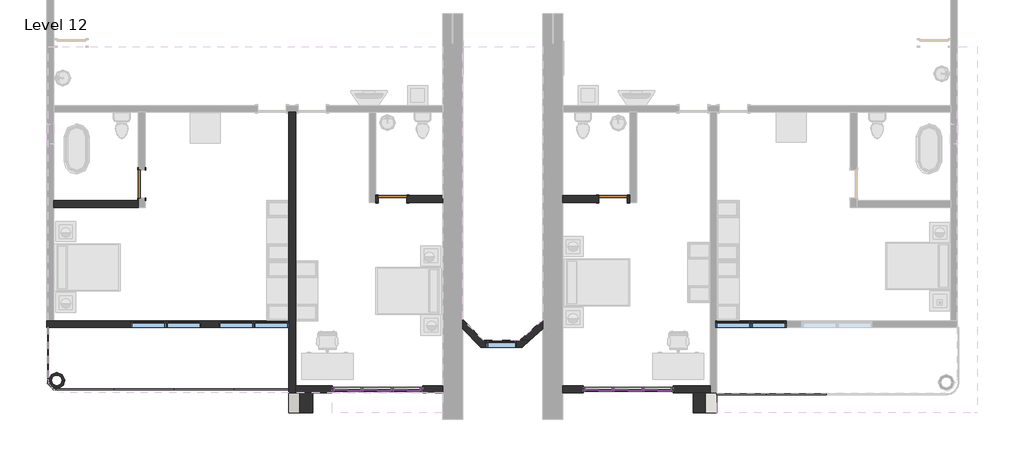
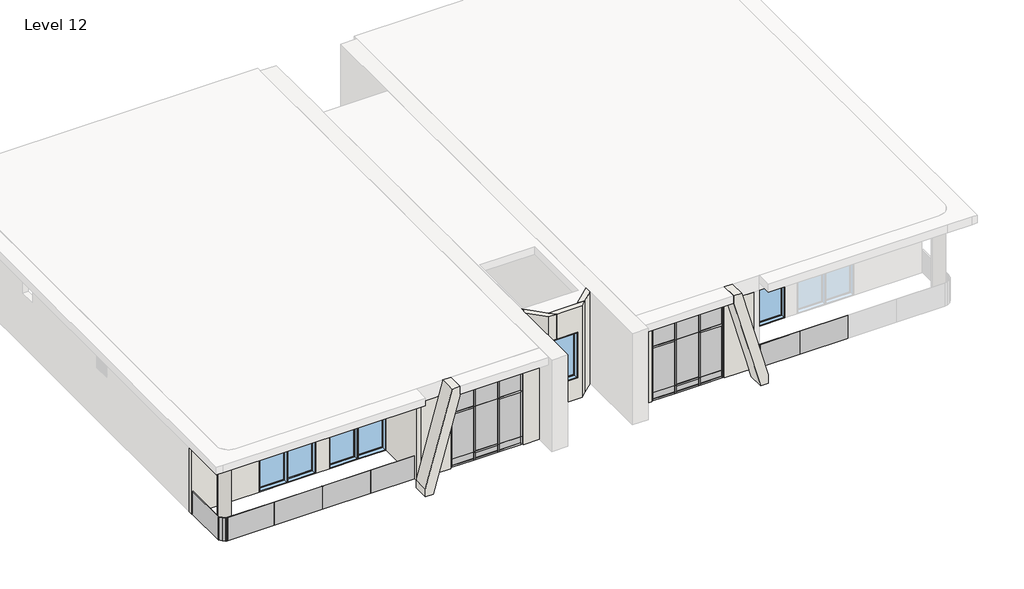
# One storey, part 1 of 3: 42 members, 29 plates, 16 walls, 7 windows, 3 doors.
"""IFC4 building model written with IfcOpenShell, lengths in millimetres."""

from ifc_helpers import new_model, si_unit, point, frame, frame_2d, origin, place, context, project, spatial, polyline, circle_curve, trimmed, segment, composite_curve, outline, extrude, faceted_brep, transform, mapped, element, save
from components import door_2703ae13, door_10fd3a06, member_c17f1be2, member_ad567e07, member_d2e7e466, member_7db1855a, member_75d1e245, member_d60e8053, member_3c3dc66a, member_2fae0574, member_410c6227, member_73c23c35, system_panel_glazed_38d54ecf, system_panel_glazed_fbb6c980, system_panel_glazed_4137532c, system_panel_glazed_6230de04, system_panel_glazed_a79f7f85, system_panel_glazed_9a5ea490, system_panel_glazed_95be5de7, system_panel_glazed_ffe51582, system_panel_glazed_8f95e3f6, system_panel_glazed_836907cd, system_panel_glazed_688a65a2, system_panel_glazed_c1a1c740, system_panel_glazed_22bcd51f, system_panel_glazed_b07a1a35, window_9a779fa2, window_1a213a25

model = new_model("IFC4")

# Units and contexts
model_context = context("Model", 3, world=origin())
ifc_project = project(units=[si_unit("LENGTHUNIT", "METRE", prefix="MILLI")], contexts=[model_context])

# Site, building, storey
site = spatial("IfcSite", under=ifc_project)
building = spatial("IfcBuilding", under=site)
storey = spatial("IfcBuildingStorey", under=building, Name="Level 12", Elevation=40233.6)

# Doors
placement = place(None, origin())
door_shape = door_2703ae13(model_context)
element("IfcDoor", 1, ObjectType="Door-Single-Panel.0001 : 34\" x 80\"", at=placement, inside=storey, context=model_context, shape_type="MappedRepresentation", body=[
    mapped(door_shape, transform((-15765.9987704, -441.9241442, 40233.6), x_axis=(0.0, -1.0, 0.0), y_axis=(1.0, 0.0, 0.0), z_axis=(0.0, 0.0, 1.0))),
])
element("IfcDoor", 2, ObjectType="Door-Single-Panel.0001 : 34\" x 80\"", at=placement, inside=storey, context=model_context, shape_type="MappedRepresentation", body=[
    mapped(door_shape, transform((-8145.9987704, -899.1241442, 40233.6), x_axis=(-1.0, 0.0, 0.0), y_axis=(0.0, -1.0, 0.0), z_axis=(0.0, 0.0, 1.0))),
])
door_2_shape = door_10fd3a06(model_context)
element("IfcDoor", 3, ObjectType="Door-Single-Panel.0001 : 34\" x 80\"", at=placement, inside=storey, context=model_context, shape_type="MappedRepresentation", body=[
    mapped(door_2_shape, transform((-1440.3987704, -899.1241442, 40233.6), x_axis=(1.0, 0.0, 0.0), y_axis=(0.0, 1.0, 0.0), z_axis=(0.0, 0.0, 1.0))),
])

# Members
member_shape = member_c17f1be2(model_context)
element("IfcMember", 4, ObjectType="Rectangular Mullion : 2.5\" x 5\" rectangular", at=placement, inside=storey, context=model_context, shape_type="MappedRepresentation", body=[
    mapped(member_shape, transform((-9911.2987704, -6690.3241442, 43281.6), x_axis=(0.0, 0.0, 1.0), y_axis=(0.0, 1.0, 0.0), z_axis=(-1.0, 0.0, 0.0))),
])
element("IfcMember", 5, ObjectType="Rectangular Mullion : 2.5\" x 5\" rectangular", at=placement, inside=storey, context=model_context, shape_type="MappedRepresentation", body=[
    mapped(member_shape, transform((-8114.2487704, -6690.3241442, 43281.6), x_axis=(0.0, 0.0, 1.0), y_axis=(0.0, 1.0, 0.0), z_axis=(-1.0, 0.0, 0.0))),
])
element("IfcMember", 6, ObjectType="Rectangular Mullion : 2.5\" x 5\" rectangular", at=placement, inside=storey, context=model_context, shape_type="MappedRepresentation", body=[
    mapped(member_shape, transform((-2291.2987704, -6690.3241442, 43281.6), x_axis=(0.0, 0.0, 1.0), y_axis=(0.0, 1.0, 0.0), z_axis=(-1.0, 0.0, 0.0))),
])
element("IfcMember", 7, ObjectType="Rectangular Mullion : 2.5\" x 5\" rectangular", at=placement, inside=storey, context=model_context, shape_type="MappedRepresentation", body=[
    mapped(member_shape, transform((-494.2487704, -6690.3241442, 43281.6), x_axis=(0.0, 0.0, 1.0), y_axis=(0.0, 1.0, 0.0), z_axis=(-1.0, 0.0, 0.0))),
])
element("IfcMember", 8, ObjectType="Rectangular Mullion : 2.5\" x 5\" rectangular", at=placement, inside=storey, context=model_context, shape_type="MappedRepresentation", body=[
    mapped(member_shape, transform((-7295.0987704, -6690.3241442, 40233.6), x_axis=(0.0, 0.0, -1.0), y_axis=(0.0, 1.0, 0.0), z_axis=(1.0, 0.0, 0.0))),
])
element("IfcMember", 9, ObjectType="Rectangular Mullion : 2.5\" x 5\" rectangular", at=placement, inside=storey, context=model_context, shape_type="MappedRepresentation", body=[
    mapped(member_shape, transform((-9092.1487704, -6690.3241442, 40233.6), x_axis=(0.0, 0.0, -1.0), y_axis=(0.0, 1.0, 0.0), z_axis=(1.0, 0.0, 0.0))),
])
element("IfcMember", 10, ObjectType="Rectangular Mullion : 2.5\" x 5\" rectangular", at=placement, inside=storey, context=model_context, shape_type="MappedRepresentation", body=[
    mapped(member_shape, transform((324.9012296, -6690.3241442, 40233.6), x_axis=(0.0, 0.0, -1.0), y_axis=(0.0, 1.0, 0.0), z_axis=(1.0, 0.0, 0.0))),
])
element("IfcMember", 11, ObjectType="Rectangular Mullion : 2.5\" x 5\" rectangular", at=placement, inside=storey, context=model_context, shape_type="MappedRepresentation", body=[
    mapped(member_shape, transform((-1472.1487704, -6690.3241442, 40233.6), x_axis=(0.0, 0.0, -1.0), y_axis=(0.0, 1.0, 0.0), z_axis=(1.0, 0.0, 0.0))),
])
member_2_shape = member_ad567e07(model_context)
element("IfcMember", 12, ObjectType="Rectangular Mullion : 2.5\" x 5\" rectangular", at=placement, inside=storey, context=model_context, shape_type="MappedRepresentation", body=[
    mapped(member_2_shape, transform((-8114.2487704, -6690.3241442, 42367.2), x_axis=(0.0, 0.0, 1.0), y_axis=(0.0, 1.0, 0.0), z_axis=(-1.0, 0.0, 0.0))),
])
element("IfcMember", 13, ObjectType="Rectangular Mullion : 2.5\" x 5\" rectangular", at=placement, inside=storey, context=model_context, shape_type="MappedRepresentation", body=[
    mapped(member_2_shape, transform((-9911.2987704, -6690.3241442, 42367.2), x_axis=(0.0, 0.0, 1.0), y_axis=(0.0, 1.0, 0.0), z_axis=(-1.0, 0.0, 0.0))),
])
element("IfcMember", 14, ObjectType="Rectangular Mullion : 2.5\" x 5\" rectangular", at=placement, inside=storey, context=model_context, shape_type="MappedRepresentation", body=[
    mapped(member_2_shape, transform((-494.2487704, -6690.3241442, 42367.2), x_axis=(0.0, 0.0, 1.0), y_axis=(0.0, 1.0, 0.0), z_axis=(-1.0, 0.0, 0.0))),
])
element("IfcMember", 15, ObjectType="Rectangular Mullion : 2.5\" x 5\" rectangular", at=placement, inside=storey, context=model_context, shape_type="MappedRepresentation", body=[
    mapped(member_2_shape, transform((-2291.2987704, -6690.3241442, 42367.2), x_axis=(0.0, 0.0, 1.0), y_axis=(0.0, 1.0, 0.0), z_axis=(-1.0, 0.0, 0.0))),
])
member_3_shape = member_d2e7e466(model_context)
element("IfcMember", 16, ObjectType="Rectangular Mullion : 2.5\" x 5\" rectangular", at=placement, inside=storey, context=model_context, shape_type="MappedRepresentation", body=[
    mapped(member_3_shape, transform((-8177.7487704, -6690.3241442, 40233.6), x_axis=(0.0, 0.0, -1.0), y_axis=(0.0, 1.0, 0.0), z_axis=(1.0, 0.0, 0.0))),
])
element("IfcMember", 17, ObjectType="Rectangular Mullion : 2.5\" x 5\" rectangular", at=placement, inside=storey, context=model_context, shape_type="MappedRepresentation", body=[
    mapped(member_3_shape, transform((-557.7487704, -6690.3241442, 40233.6), x_axis=(0.0, 0.0, -1.0), y_axis=(0.0, 1.0, 0.0), z_axis=(1.0, 0.0, 0.0))),
])
member_4_shape = member_7db1855a(model_context)
element("IfcMember", 18, ObjectType="Rectangular Mullion : 2.5\" x 5\" rectangular", at=placement, inside=storey, context=model_context, shape_type="MappedRepresentation", body=[
    mapped(member_4_shape, transform((-9028.6487704, -6690.3241442, 40538.4), x_axis=(0.0, 0.0, 1.0), y_axis=(0.0, 1.0, 0.0), z_axis=(-1.0, 0.0, 0.0))),
])
element("IfcMember", 19, ObjectType="Rectangular Mullion : 2.5\" x 5\" rectangular", at=placement, inside=storey, context=model_context, shape_type="MappedRepresentation", body=[
    mapped(member_4_shape, transform((-1408.6487704, -6690.3241442, 40538.4), x_axis=(0.0, 0.0, 1.0), y_axis=(0.0, 1.0, 0.0), z_axis=(-1.0, 0.0, 0.0))),
])
element("IfcMember", 20, ObjectType="Rectangular Mullion : 2.5\" x 5\" rectangular", at=placement, inside=storey, context=model_context, shape_type="MappedRepresentation", body=[
    mapped(member_3_shape, transform((-9028.6487704, -6690.3241442, 43281.6), x_axis=(0.0, 0.0, 1.0), y_axis=(0.0, 1.0, 0.0), z_axis=(-1.0, 0.0, 0.0))),
])
element("IfcMember", 21, ObjectType="Rectangular Mullion : 2.5\" x 5\" rectangular", at=placement, inside=storey, context=model_context, shape_type="MappedRepresentation", body=[
    mapped(member_3_shape, transform((-1408.6487704, -6690.3241442, 43281.6), x_axis=(0.0, 0.0, 1.0), y_axis=(0.0, 1.0, 0.0), z_axis=(-1.0, 0.0, 0.0))),
])
member_5_shape = member_75d1e245(model_context)
element("IfcMember", 22, ObjectType="Rectangular Mullion : 2.5\" x 5\" rectangular", at=placement, inside=storey, context=model_context, shape_type="MappedRepresentation", body=[
    mapped(member_5_shape, transform((-8145.9987704, -6690.3241442, 40233.6), x_axis=(-1.0, 0.0, 0.0), y_axis=(0.0, 1.0, 0.0), z_axis=(0.0, 0.0, -1.0))),
])
element("IfcMember", 23, ObjectType="Rectangular Mullion : 2.5\" x 5\" rectangular", at=placement, inside=storey, context=model_context, shape_type="MappedRepresentation", body=[
    mapped(member_5_shape, transform((-9060.3987704, -6690.3241442, 40233.6), x_axis=(-1.0, 0.0, 0.0), y_axis=(0.0, 1.0, 0.0), z_axis=(0.0, 0.0, -1.0))),
])
element("IfcMember", 24, ObjectType="Rectangular Mullion : 2.5\" x 5\" rectangular", at=placement, inside=storey, context=model_context, shape_type="MappedRepresentation", body=[
    mapped(member_5_shape, transform((-525.9987704, -6690.3241442, 40233.6), x_axis=(-1.0, 0.0, 0.0), y_axis=(0.0, 1.0, 0.0), z_axis=(0.0, 0.0, -1.0))),
])
element("IfcMember", 25, ObjectType="Rectangular Mullion : 2.5\" x 5\" rectangular", at=placement, inside=storey, context=model_context, shape_type="MappedRepresentation", body=[
    mapped(member_5_shape, transform((-1440.3987704, -6690.3241442, 40233.6), x_axis=(-1.0, 0.0, 0.0), y_axis=(0.0, 1.0, 0.0), z_axis=(0.0, 0.0, -1.0))),
])
member_6_shape = member_d60e8053(model_context)
element("IfcMember", 26, ObjectType="Rectangular Mullion : 2.5\" x 5\" rectangular", at=placement, inside=storey, context=model_context, shape_type="MappedRepresentation", body=[
    mapped(member_6_shape, transform((-8145.9987704, -6690.3241442, 40538.4), x_axis=(-1.0, 0.0, 0.0), y_axis=(0.0, 1.0, 0.0), z_axis=(0.0, 0.0, -1.0))),
])
element("IfcMember", 27, ObjectType="Rectangular Mullion : 2.5\" x 5\" rectangular", at=placement, inside=storey, context=model_context, shape_type="MappedRepresentation", body=[
    mapped(member_6_shape, transform((-9060.3987704, -6690.3241442, 40538.4), x_axis=(-1.0, 0.0, 0.0), y_axis=(0.0, 1.0, 0.0), z_axis=(0.0, 0.0, -1.0))),
])
element("IfcMember", 28, ObjectType="Rectangular Mullion : 2.5\" x 5\" rectangular", at=placement, inside=storey, context=model_context, shape_type="MappedRepresentation", body=[
    mapped(member_6_shape, transform((-525.9987704, -6690.3241442, 40538.4), x_axis=(-1.0, 0.0, 0.0), y_axis=(0.0, 1.0, 0.0), z_axis=(0.0, 0.0, -1.0))),
])
element("IfcMember", 29, ObjectType="Rectangular Mullion : 2.5\" x 5\" rectangular", at=placement, inside=storey, context=model_context, shape_type="MappedRepresentation", body=[
    mapped(member_6_shape, transform((-1440.3987704, -6690.3241442, 40538.4), x_axis=(-1.0, 0.0, 0.0), y_axis=(0.0, 1.0, 0.0), z_axis=(0.0, 0.0, -1.0))),
])
member_7_shape = member_3c3dc66a(model_context)
element("IfcMember", 30, ObjectType="Rectangular Mullion : 2.5\" x 5\" rectangular", at=placement, inside=storey, context=model_context, shape_type="MappedRepresentation", body=[
    mapped(member_7_shape, transform((-9974.7987704, -6690.3241442, 40233.6), x_axis=(-1.0, 0.0, 0.0), y_axis=(0.0, 1.0, 0.0), z_axis=(0.0, 0.0, -1.0))),
])
element("IfcMember", 31, ObjectType="Rectangular Mullion : 2.5\" x 5\" rectangular", at=placement, inside=storey, context=model_context, shape_type="MappedRepresentation", body=[
    mapped(member_7_shape, transform((-2354.7987704, -6690.3241442, 40233.6), x_axis=(-1.0, 0.0, 0.0), y_axis=(0.0, 1.0, 0.0), z_axis=(0.0, 0.0, -1.0))),
])
member_8_shape = member_2fae0574(model_context)
element("IfcMember", 32, ObjectType="Rectangular Mullion : 2.5\" x 5\" rectangular", at=placement, inside=storey, context=model_context, shape_type="MappedRepresentation", body=[
    mapped(member_8_shape, transform((-9974.7987704, -6690.3241442, 40538.4), x_axis=(-1.0, 0.0, 0.0), y_axis=(0.0, 1.0, 0.0), z_axis=(0.0, 0.0, -1.0))),
])
element("IfcMember", 33, ObjectType="Rectangular Mullion : 2.5\" x 5\" rectangular", at=placement, inside=storey, context=model_context, shape_type="MappedRepresentation", body=[
    mapped(member_8_shape, transform((-2354.7987704, -6690.3241442, 40538.4), x_axis=(-1.0, 0.0, 0.0), y_axis=(0.0, 1.0, 0.0), z_axis=(0.0, 0.0, -1.0))),
])
element("IfcMember", 34, ObjectType="Rectangular Mullion : 2.5\" x 5\" rectangular", at=placement, inside=storey, context=model_context, shape_type="MappedRepresentation", body=[
    mapped(member_8_shape, transform((-7231.5987704, -6690.3241442, 42367.2), x_axis=(1.0, 0.0, 0.0), y_axis=(0.0, 1.0, 0.0), z_axis=(0.0, 0.0, 1.0))),
])
element("IfcMember", 35, ObjectType="Rectangular Mullion : 2.5\" x 5\" rectangular", at=placement, inside=storey, context=model_context, shape_type="MappedRepresentation", body=[
    mapped(member_8_shape, transform((388.4012296, -6690.3241442, 42367.2), x_axis=(1.0, 0.0, 0.0), y_axis=(0.0, 1.0, 0.0), z_axis=(0.0, 0.0, 1.0))),
])
element("IfcMember", 36, ObjectType="Rectangular Mullion : 2.5\" x 5\" rectangular", at=placement, inside=storey, context=model_context, shape_type="MappedRepresentation", body=[
    mapped(member_7_shape, transform((-7231.5987704, -6690.3241442, 40538.4), x_axis=(1.0, 0.0, 0.0), y_axis=(0.0, 1.0, 0.0), z_axis=(0.0, 0.0, 1.0))),
])
element("IfcMember", 37, ObjectType="Rectangular Mullion : 2.5\" x 5\" rectangular", at=placement, inside=storey, context=model_context, shape_type="MappedRepresentation", body=[
    mapped(member_7_shape, transform((388.4012296, -6690.3241442, 40538.4), x_axis=(1.0, 0.0, 0.0), y_axis=(0.0, 1.0, 0.0), z_axis=(0.0, 0.0, 1.0))),
])
member_9_shape = member_410c6227(model_context)
element("IfcMember", 38, ObjectType="Rectangular Mullion : 2.5\" x 5\" rectangular", at=placement, inside=storey, context=model_context, shape_type="MappedRepresentation", body=[
    mapped(member_9_shape, transform((-8145.9987704, -6690.3241442, 42367.2), x_axis=(-1.0, 0.0, 0.0), y_axis=(0.0, 1.0, 0.0), z_axis=(0.0, 0.0, -1.0))),
])
element("IfcMember", 39, ObjectType="Rectangular Mullion : 2.5\" x 5\" rectangular", at=placement, inside=storey, context=model_context, shape_type="MappedRepresentation", body=[
    mapped(member_9_shape, transform((-9060.3987704, -6690.3241442, 42367.2), x_axis=(-1.0, 0.0, 0.0), y_axis=(0.0, 1.0, 0.0), z_axis=(0.0, 0.0, -1.0))),
])
element("IfcMember", 40, ObjectType="Rectangular Mullion : 2.5\" x 5\" rectangular", at=placement, inside=storey, context=model_context, shape_type="MappedRepresentation", body=[
    mapped(member_9_shape, transform((-525.9987704, -6690.3241442, 42367.2), x_axis=(-1.0, 0.0, 0.0), y_axis=(0.0, 1.0, 0.0), z_axis=(0.0, 0.0, -1.0))),
])
element("IfcMember", 41, ObjectType="Rectangular Mullion : 2.5\" x 5\" rectangular", at=placement, inside=storey, context=model_context, shape_type="MappedRepresentation", body=[
    mapped(member_9_shape, transform((-1440.3987704, -6690.3241442, 42367.2), x_axis=(-1.0, 0.0, 0.0), y_axis=(0.0, 1.0, 0.0), z_axis=(0.0, 0.0, -1.0))),
])
member_10_shape = member_73c23c35(model_context)
element("IfcMember", 42, ObjectType="Rectangular Mullion : 2.5\" x 5\" rectangular", at=placement, inside=storey, context=model_context, shape_type="MappedRepresentation", body=[
    mapped(member_10_shape, transform((-7231.5987704, -6690.3241442, 43281.6), x_axis=(1.0, 0.0, 0.0), y_axis=(0.0, 1.0, 0.0), z_axis=(0.0, 0.0, 1.0))),
])
element("IfcMember", 43, ObjectType="Rectangular Mullion : 2.5\" x 5\" rectangular", at=placement, inside=storey, context=model_context, shape_type="MappedRepresentation", body=[
    mapped(member_10_shape, transform((388.4012296, -6690.3241442, 43281.6), x_axis=(1.0, 0.0, 0.0), y_axis=(0.0, 1.0, 0.0), z_axis=(0.0, 0.0, 1.0))),
])
element("IfcMember", 44, ObjectType="Rectangular Mullion : 2.5\" x 5\" rectangular", at=placement, inside=storey, context=model_context, shape_type="MappedRepresentation", body=[
    mapped(member_10_shape, transform((-9974.7987704, -6690.3241442, 42367.2), x_axis=(-1.0, 0.0, 0.0), y_axis=(0.0, 1.0, 0.0), z_axis=(0.0, 0.0, -1.0))),
])
element("IfcMember", 45, ObjectType="Rectangular Mullion : 2.5\" x 5\" rectangular", at=placement, inside=storey, context=model_context, shape_type="MappedRepresentation", body=[
    mapped(member_10_shape, transform((-2354.7987704, -6690.3241442, 42367.2), x_axis=(-1.0, 0.0, 0.0), y_axis=(0.0, 1.0, 0.0), z_axis=(0.0, 0.0, -1.0))),
])

# Plates
system_panel_glazed_shape = system_panel_glazed_38d54ecf(model_context)
element("IfcPlate", 46, ObjectType="System Panel : Glazed", at=placement, inside=storey, context=model_context, shape_type="MappedRepresentation", body=[
    mapped(system_panel_glazed_shape, transform((-8603.1987704, -6690.3241442, 40570.15), x_axis=(-1.0, 0.0, 0.0), y_axis=(0.0, -1.0, 0.0), z_axis=(0.0, 0.0, 1.0))),
])
element("IfcPlate", 47, ObjectType="System Panel : Glazed", at=placement, inside=storey, context=model_context, shape_type="MappedRepresentation", body=[
    mapped(system_panel_glazed_shape, transform((-983.1987704, -6690.3241442, 40570.15), x_axis=(-1.0, 0.0, 0.0), y_axis=(0.0, -1.0, 0.0), z_axis=(0.0, 0.0, 1.0))),
])
system_panel_glazed_2_shape = system_panel_glazed_fbb6c980(model_context)
element("IfcPlate", 48, ObjectType="System Panel : Glazed", at=placement, inside=storey, context=model_context, shape_type="MappedRepresentation", body=[
    mapped(system_panel_glazed_2_shape, transform((-8603.1987704, -6690.3241442, 40297.1), x_axis=(-1.0, 0.0, 0.0), y_axis=(0.0, -1.0, 0.0), z_axis=(0.0, 0.0, 1.0))),
])
element("IfcPlate", 49, ObjectType="System Panel : Glazed", at=placement, inside=storey, context=model_context, shape_type="MappedRepresentation", body=[
    mapped(system_panel_glazed_2_shape, transform((-983.1987704, -6690.3241442, 40297.1), x_axis=(-1.0, 0.0, 0.0), y_axis=(0.0, -1.0, 0.0), z_axis=(0.0, 0.0, 1.0))),
])
system_panel_glazed_3_shape = system_panel_glazed_4137532c(model_context)
element("IfcPlate", 50, ObjectType="System Panel : Glazed", at=placement, inside=storey, context=model_context, shape_type="MappedRepresentation", body=[
    mapped(system_panel_glazed_3_shape, transform((-7704.6737704, -6690.3241442, 40297.1), x_axis=(-1.0, 0.0, 0.0), y_axis=(0.0, -1.0, 0.0), z_axis=(0.0, 0.0, 1.0))),
])
element("IfcPlate", 51, ObjectType="System Panel : Glazed", at=placement, inside=storey, context=model_context, shape_type="MappedRepresentation", body=[
    mapped(system_panel_glazed_3_shape, transform((-9501.7237704, -6690.3241442, 40297.1), x_axis=(-1.0, 0.0, 0.0), y_axis=(0.0, -1.0, 0.0), z_axis=(0.0, 0.0, 1.0))),
])
element("IfcPlate", 52, ObjectType="System Panel : Glazed", at=placement, inside=storey, context=model_context, shape_type="MappedRepresentation", body=[
    mapped(system_panel_glazed_3_shape, transform((-84.6737704, -6690.3241442, 40297.1), x_axis=(-1.0, 0.0, 0.0), y_axis=(0.0, -1.0, 0.0), z_axis=(0.0, 0.0, 1.0))),
])
element("IfcPlate", 53, ObjectType="System Panel : Glazed", at=placement, inside=storey, context=model_context, shape_type="MappedRepresentation", body=[
    mapped(system_panel_glazed_3_shape, transform((-1881.7237704, -6690.3241442, 40297.1), x_axis=(-1.0, 0.0, 0.0), y_axis=(0.0, -1.0, 0.0), z_axis=(0.0, 0.0, 1.0))),
])
system_panel_glazed_4_shape = system_panel_glazed_6230de04(model_context)
element("IfcPlate", 54, ObjectType="System Panel : Glazed", at=placement, inside=storey, context=model_context, shape_type="MappedRepresentation", body=[
    mapped(system_panel_glazed_4_shape, transform((-7704.6737704, -6690.3241442, 40538.4), x_axis=(-1.0, 0.0, 0.0), y_axis=(0.0, -1.0, 0.0), z_axis=(0.0, 0.0, 1.0))),
])
element("IfcPlate", 55, ObjectType="System Panel : Glazed", at=placement, inside=storey, context=model_context, shape_type="MappedRepresentation", body=[
    mapped(system_panel_glazed_4_shape, transform((-9501.7237704, -6690.3241442, 40538.4), x_axis=(-1.0, 0.0, 0.0), y_axis=(0.0, -1.0, 0.0), z_axis=(0.0, 0.0, 1.0))),
])
element("IfcPlate", 56, ObjectType="System Panel : Glazed", at=placement, inside=storey, context=model_context, shape_type="MappedRepresentation", body=[
    mapped(system_panel_glazed_4_shape, transform((-84.6737704, -6690.3241442, 40538.4), x_axis=(-1.0, 0.0, 0.0), y_axis=(0.0, -1.0, 0.0), z_axis=(0.0, 0.0, 1.0))),
])
element("IfcPlate", 57, ObjectType="System Panel : Glazed", at=placement, inside=storey, context=model_context, shape_type="MappedRepresentation", body=[
    mapped(system_panel_glazed_4_shape, transform((-1881.7237704, -6690.3241442, 40538.4), x_axis=(-1.0, 0.0, 0.0), y_axis=(0.0, -1.0, 0.0), z_axis=(0.0, 0.0, 1.0))),
])
system_panel_glazed_5_shape = system_panel_glazed_a79f7f85(model_context)
element("IfcPlate", 58, ObjectType="System Panel : Glazed", at=placement, inside=storey, context=model_context, shape_type="MappedRepresentation", body=[
    mapped(system_panel_glazed_5_shape, transform((-7704.6737704, -6690.3241442, 42398.95), x_axis=(-1.0, 0.0, 0.0), y_axis=(0.0, -1.0, 0.0), z_axis=(0.0, 0.0, 1.0))),
])
element("IfcPlate", 59, ObjectType="System Panel : Glazed", at=placement, inside=storey, context=model_context, shape_type="MappedRepresentation", body=[
    mapped(system_panel_glazed_5_shape, transform((-9501.7237704, -6690.3241442, 42398.95), x_axis=(-1.0, 0.0, 0.0), y_axis=(0.0, -1.0, 0.0), z_axis=(0.0, 0.0, 1.0))),
])
element("IfcPlate", 60, ObjectType="System Panel : Glazed", at=placement, inside=storey, context=model_context, shape_type="MappedRepresentation", body=[
    mapped(system_panel_glazed_5_shape, transform((-84.6737704, -6690.3241442, 42398.95), x_axis=(-1.0, 0.0, 0.0), y_axis=(0.0, -1.0, 0.0), z_axis=(0.0, 0.0, 1.0))),
])
element("IfcPlate", 61, ObjectType="System Panel : Glazed", at=placement, inside=storey, context=model_context, shape_type="MappedRepresentation", body=[
    mapped(system_panel_glazed_5_shape, transform((-1881.7237704, -6690.3241442, 42398.95), x_axis=(-1.0, 0.0, 0.0), y_axis=(0.0, -1.0, 0.0), z_axis=(0.0, 0.0, 1.0))),
])
system_panel_glazed_6_shape = system_panel_glazed_9a5ea490(model_context)
element("IfcPlate", 62, ObjectType="System Panel : Glazed", at=placement, inside=storey, context=model_context, shape_type="MappedRepresentation", body=[
    mapped(system_panel_glazed_6_shape, transform((-8603.1987704, -6690.3241442, 42367.2), x_axis=(-1.0, 0.0, 0.0), y_axis=(0.0, -1.0, 0.0), z_axis=(0.0, 0.0, 1.0))),
])
element("IfcPlate", 63, ObjectType="System Panel : Glazed", at=placement, inside=storey, context=model_context, shape_type="MappedRepresentation", body=[
    mapped(system_panel_glazed_6_shape, transform((-983.1987704, -6690.3241442, 42367.2), x_axis=(-1.0, 0.0, 0.0), y_axis=(0.0, -1.0, 0.0), z_axis=(0.0, 0.0, 1.0))),
])
system_panel_glazed_7_shape = system_panel_glazed_95be5de7(model_context)
element("IfcPlate", 64, ObjectType="System Panel : Glazed", at=placement, inside=storey, context=model_context, shape_type="MappedRepresentation", body=[
    mapped(system_panel_glazed_7_shape, transform((-15707.2305745, -6723.6923401, 40233.6), x_axis=(1.0, 0.0, 0.0), y_axis=(0.0, 1.0, 0.0), z_axis=(0.0, 0.0, 1.0))),
])
element("IfcPlate", 65, ObjectType="System Panel : Glazed", at=placement, inside=storey, context=model_context, shape_type="MappedRepresentation", body=[
    mapped(system_panel_glazed_7_shape, transform((-13878.4305745, -6723.6923401, 40233.6), x_axis=(1.0, 0.0, 0.0), y_axis=(0.0, 1.0, 0.0), z_axis=(0.0, 0.0, 1.0))),
])
element("IfcPlate", 66, ObjectType="System Panel : Glazed", at=placement, inside=storey, context=model_context, shape_type="MappedRepresentation", body=[
    mapped(system_panel_glazed_7_shape, transform((4129.1120092, -6810.4133646, 40233.6), x_axis=(-1.0, 0.0, 0.0), y_axis=(0.0, -1.0, 0.0), z_axis=(0.0, 0.0, 1.0))),
])
system_panel_glazed_8_shape = system_panel_glazed_ffe51582(model_context)
element("IfcPlate", 67, ObjectType="System Panel : Glazed", at=placement, inside=storey, context=model_context, shape_type="MappedRepresentation", body=[
    mapped(system_panel_glazed_8_shape, transform((-18451.9713429, -6722.1515718, 40233.6), x_axis=(0.7071067811865462, -0.7071067811865488, 0.0), y_axis=(0.7071067811865488, 0.7071067811865462, 0.0), z_axis=(0.0, 0.0, 1.0))),
])
system_panel_glazed_9_shape = system_panel_glazed_8f95e3f6(model_context)
element("IfcPlate", 68, ObjectType="System Panel : Glazed", at=placement, inside=storey, context=model_context, shape_type="MappedRepresentation", body=[
    mapped(system_panel_glazed_9_shape, transform((-18648.8987704, -5667.9741442, 40233.6), x_axis=(0.0, -1.0, 0.0), y_axis=(1.0, 0.0, 0.0), z_axis=(0.0, 0.0, 1.0))),
])
system_panel_glazed_10_shape = system_panel_glazed_836907cd(model_context)
element("IfcPlate", 69, ObjectType="System Panel : Glazed", at=placement, inside=storey, context=model_context, shape_type="MappedRepresentation", body=[
    mapped(system_panel_glazed_10_shape, transform((-18418.6805745, -6723.6923401, 40233.6), x_axis=(1.0, 0.0, 0.0), y_axis=(0.0, 1.0, 0.0), z_axis=(0.0, 0.0, 1.0))),
])
system_panel_glazed_11_shape = system_panel_glazed_688a65a2(model_context)
element("IfcPlate", 70, ObjectType="System Panel : Glazed", at=placement, inside=storey, context=model_context, shape_type="MappedRepresentation", body=[
    mapped(system_panel_glazed_11_shape, transform((-12129.8146725, -6723.6923401, 40233.6), x_axis=(1.0, 0.0, 0.0), y_axis=(0.0, 1.0, 0.0), z_axis=(0.0, 0.0, 1.0))),
])
system_panel_glazed_12_shape = system_panel_glazed_c1a1c740(model_context)
element("IfcPlate", 71, ObjectType="System Panel : Glazed", at=placement, inside=storey, context=model_context, shape_type="MappedRepresentation", body=[
    mapped(system_panel_glazed_12_shape, transform((-17504.2805745, -6723.6923401, 40233.6), x_axis=(1.0, 0.0, 0.0), y_axis=(0.0, 1.0, 0.0), z_axis=(0.0, 0.0, 1.0))),
])
system_panel_glazed_13_shape = system_panel_glazed_22bcd51f(model_context)
element("IfcPlate", 72, ObjectType="System Panel : Glazed", at=placement, inside=storey, context=model_context, shape_type="MappedRepresentation", body=[
    mapped(system_panel_glazed_13_shape, transform((-18600.0521056, -6574.070809, 40233.6), x_axis=(0.7071067811865462, -0.7071067811865488, 0.0), y_axis=(0.7071067811865488, 0.7071067811865462, 0.0), z_axis=(0.0, 0.0, 1.0))),
])
element("IfcPlate", 73, ObjectType="System Panel : Glazed", at=placement, inside=storey, context=model_context, shape_type="MappedRepresentation", body=[
    mapped(system_panel_glazed_13_shape, transform((-18502.3587761, -6671.7641386, 40233.6), x_axis=(0.7071067811865462, -0.7071067811865488, 0.0), y_axis=(0.7071067811865488, 0.7071067811865462, 0.0), z_axis=(0.0, 0.0, 1.0))),
])
system_panel_glazed_14_shape = system_panel_glazed_b07a1a35(model_context)
element("IfcPlate", 74, ObjectType="System Panel : Glazed", at=placement, inside=storey, context=model_context, shape_type="MappedRepresentation", body=[
    mapped(system_panel_glazed_14_shape, transform((2462.0968143, -6810.4133646, 40233.6), x_axis=(-1.0, 0.0, 0.0), y_axis=(0.0, -1.0, 0.0), z_axis=(0.0, 0.0, 1.0))),
])

# Walls
element("IfcWall", 75, ObjectType="Generic - 3\" green 2", at=placement, inside=storey, context=model_context, shape_type="SweptSolid", body=[
    extrude(outline(composite_curve([segment(polyline([(-18518.7237704, -6418.8616442), (-18594.9237704, -6418.8616442)]), True, "CONTINUOUS"), segment(trimmed(circle_curve(frame_2d((-18353.6237704, -6418.8616442)), 241.3), [point((-18594.9237704, -6418.8616442))], [point((-18112.3237704, -6418.8616442))], False, "CARTESIAN"), True, "CONTINUOUS"), segment(polyline([(-18112.3237704, -6418.8616442), (-18188.5237704, -6418.8616442)]), True, "CONTINUOUS"), segment(trimmed(circle_curve(frame_2d((-18353.6237704, -6418.8616442)), 165.1), [point((-18188.5237704, -6418.8616442))], [point((-18518.7237704, -6418.8616442))], True, "CARTESIAN"), True, "CONTINUOUS")], self_intersect=False)), frame((0.0, 0.0, 40233.6), z_axis=(0.0, 0.0, 1.0), x_axis=(1.0, 0.0, 0.0)), (0.0, 0.0, 1.0), 3048.0),
])
element("IfcWall", 76, ObjectType="Generic - 3\" green 2", at=placement, inside=storey, context=model_context, shape_type="SweptSolid", body=[
    extrude(outline(composite_curve([segment(polyline([(-18188.5237704, -6418.8616442), (-18112.3237704, -6418.8616442)]), True, "CONTINUOUS"), segment(trimmed(circle_curve(frame_2d((-18353.6237704, -6418.8616442)), 241.3), [point((-18112.3237704, -6418.8616442))], [point((-18594.9237704, -6418.8616442))], False, "CARTESIAN"), True, "CONTINUOUS"), segment(polyline([(-18594.9237704, -6418.8616442), (-18518.7237704, -6418.8616442)]), True, "CONTINUOUS"), segment(trimmed(circle_curve(frame_2d((-18353.6237704, -6418.8616442)), 165.1), [point((-18518.7237704, -6418.8616442))], [point((-18188.5237704, -6418.8616442))], True, "CARTESIAN"), True, "CONTINUOUS")], self_intersect=False)), frame((0.0, 0.0, 40233.6), z_axis=(0.0, 0.0, 1.0), x_axis=(1.0, 0.0, 0.0)), (0.0, 0.0, 1.0), 3048.0),
])
element("IfcWall", 77, ObjectType="Generic - 8\" cream", at=placement, inside=storey, context=model_context, shape_type="Brep", body=[
    faceted_brep([(-11295.5987704, 1742.4758558, 40233.6), (-11295.5987704, -6791.9241442, 40233.6), (-11295.5987704, -6791.9241442, 43281.6), (-11295.5987704, -4810.7241442, 43281.6), (-11295.5987704, -4607.5241442, 43281.6), (-11295.5987704, 1742.4758558, 43281.6), (-11092.3987704, 1742.4758558, 40233.6), (-11092.3987704, 1742.4758558, 43281.6), (-11092.3987704, -6588.7241442, 43281.6), (-11092.3987704, -6791.9241442, 43281.6), (-11092.3987704, -6791.9241442, 40233.6), (-11092.3987704, -6588.7241442, 40233.6)], [[[0, 1, 2, 3, 4, 5]], [[6, 7, 8, 9, 10, 11]], [[1, 0, 6, 11, 10]], [[5, 4, 3, 2, 9, 8, 7]], [[0, 5, 7, 6]], [[2, 1, 10, 9]]]),
])
element("IfcWall", 78, ObjectType="Generic - 8\" cream", at=placement, inside=storey, context=model_context, shape_type="SweptSolid", body=[
    extrude(outline(polyline([(-18445.6987704, -949.9241442), (-15867.5987704, -949.9241442), (-15867.5987704, -1153.1241442), (-18445.6987704, -1153.1241442), (-18445.6987704, -949.9241442)])), frame((0.0, 0.0, 40233.6), z_axis=(0.0, 0.0, 1.0), x_axis=(1.0, 0.0, 0.0)), (0.0, 0.0, 1.0), 3048.0),
])
element("IfcWall", 79, ObjectType="Generic - 8\" cream", at=placement, inside=storey, context=model_context, shape_type="SweptSolid", body=[
    extrude(outline(polyline([(43281.6, -6621.9987704), (43281.6, -8653.9987704), (40233.6, -8653.9987704), (40233.6, -8577.7987704), (42265.6, -8577.7987704), (42265.6, -7714.1987704), (40233.6, -7714.1987704), (40233.6, -6621.9987704), (43281.6, -6621.9987704)])), frame((0.0, -1000.7241442, 0.0), z_axis=(0.0, 1.0, 0.0), x_axis=(0.0, 0.0, 1.0)), (0.0, 0.0, 1.0), 203.2),
])
element("IfcWall", 80, ObjectType="Generic - 8\" cream", at=placement, inside=storey, context=model_context, shape_type="Brep", body=[
    faceted_brep([(-18648.8987704, -4607.5241442, 43281.6), (-18445.6987704, -4607.5241442, 43281.6), (-11295.5987704, -4607.5241442, 43281.6), (-11295.5987704, -4607.5241442, 42976.8), (-13429.1987704, -4607.5241442, 42976.8), (-13429.1987704, -4607.5241442, 40233.6), (-13962.5987704, -4607.5241442, 40233.6), (-13962.5987704, -4607.5241442, 42976.8), (-16096.1987704, -4607.5241442, 42976.8), (-16096.1987704, -4607.5241442, 40233.6), (-18445.6987704, -4607.5241442, 40233.6), (-18648.8987704, -4607.5241442, 40233.6), (-11295.5987704, -4810.7241442, 43281.6), (-18648.8987704, -4810.7241442, 43281.6), (-18648.8987704, -4810.7241442, 40233.6), (-16096.1987704, -4810.7241442, 40233.6), (-16096.1987704, -4810.7241442, 42976.8), (-13962.5987704, -4810.7241442, 42976.8), (-13962.5987704, -4810.7241442, 40233.6), (-13429.1987704, -4810.7241442, 40233.6), (-13429.1987704, -4810.7241442, 42976.8), (-11295.5987704, -4810.7241442, 42976.8)], [[[0, 1, 2, 3, 4, 5, 6, 7, 8, 9, 10, 11]], [[12, 13, 14, 15, 16, 17, 18, 19, 20, 21]], [[14, 11, 10, 9, 15]], [[5, 19, 18, 6]], [[2, 1, 0, 13, 12]], [[2, 12, 21, 3]], [[0, 11, 14, 13]], [[3, 21, 20, 4]], [[4, 20, 19, 5]], [[17, 7, 6, 18]], [[7, 17, 16, 8]], [[8, 16, 15, 9]]]),
])
element("IfcWall", 81, ObjectType="Generic - 8\" cream", at=placement, inside=storey, context=model_context, shape_type="SweptSolid", body=[
    extrude(outline(polyline([(43281.6, -932.3987704), (43281.6, -2964.3987704), (40233.6, -2964.3987704), (40233.6, -1872.1987704), (42265.6, -1872.1987704), (42265.6, -1008.5987704), (40233.6, -1008.5987704), (40233.6, -932.3987704), (43281.6, -932.3987704)])), frame((0.0, -1000.7241442, 0.0), z_axis=(0.0, 1.0, 0.0), x_axis=(0.0, 0.0, 1.0)), (0.0, 0.0, 1.0), 203.2),
])
element("IfcWall", 82, ObjectType="Generic - 8\" cream", at=placement, inside=storey, context=model_context, shape_type="SweptSolid", body=[
    extrude(outline(polyline([(388.4012296, -6588.7241442), (1506.0012296, -6588.7241442), (1506.0012296, -6791.9241442), (388.4012296, -6791.9241442), (388.4012296, -6588.7241442)])), frame((0.0, 0.0, 40233.6), z_axis=(0.0, 0.0, 1.0), x_axis=(1.0, 0.0, 0.0)), (0.0, 0.0, 1.0), 3048.0),
])
element("IfcWall", 83, ObjectType="Generic - 8\" cream", at=placement, inside=storey, context=model_context, shape_type="SweptSolid", body=[
    extrude(outline(polyline([(-2354.7987704, -6791.9241442), (-2964.3987704, -6791.9241442), (-2964.3987704, -6588.7241442), (-2354.7987704, -6588.7241442), (-2354.7987704, -6791.9241442)])), frame((0.0, 0.0, 40233.6), z_axis=(0.0, 0.0, 1.0), x_axis=(1.0, 0.0, 0.0)), (0.0, 0.0, 1.0), 3048.0),
])
element("IfcWall", 84, ObjectType="Generic - 8\" cream", at=placement, inside=storey, context=model_context, shape_type="SweptSolid", body=[
    extrude(outline(polyline([(-9974.7987704, -6791.9241442), (-11092.3987704, -6791.9241442), (-11092.3987704, -6588.7241442), (-9974.7987704, -6588.7241442), (-9974.7987704, -6791.9241442)])), frame((0.0, 0.0, 40233.6), z_axis=(0.0, 0.0, 1.0), x_axis=(1.0, 0.0, 0.0)), (0.0, 0.0, 1.0), 3048.0),
])
element("IfcWall", 85, ObjectType="Generic - 8\" cream", at=placement, inside=storey, context=model_context, shape_type="SweptSolid", body=[
    extrude(outline(polyline([(-7231.5987704, -6588.7241442), (-6621.9987704, -6588.7241442), (-6621.9987704, -6791.9241442), (-7231.5987704, -6791.9241442), (-7231.5987704, -6588.7241442)])), frame((0.0, 0.0, 40233.6), z_axis=(0.0, 0.0, 1.0), x_axis=(1.0, 0.0, 0.0)), (0.0, 0.0, 1.0), 3048.0),
])
element("IfcWall", 86, ObjectType="Generic - 8\" green", at=placement, inside=storey, context=model_context, shape_type="Brep", body=[
    faceted_brep([(-6012.3987704, -4852.8082422, 40233.6), (-5458.7044276, -5406.502585, 40233.6), (-5458.7044276, -5406.502585, 43891.2), (-6012.3987704, -4852.8082422, 43891.2), (-5171.3362318, -5406.502585, 40233.6), (-5374.5362318, -5203.302585, 40233.6), (-6012.3987704, -4565.4400463, 40233.6), (-6012.3987704, -4565.4400463, 43891.2), (-5374.5362318, -5203.302585, 43891.2), (-5171.3362318, -5406.502585, 43891.2), (-5171.3362318, -5406.502585, 42900.6), (-5289.4901401, -5288.3486766, 42900.6), (-5289.4901401, -5288.3486766, 41071.8), (-5171.3362318, -5406.502585, 41071.8), (-5289.4901401, -5406.502585, 41071.8), (-5289.4901401, -5406.502585, 42900.6)], [[[0, 1, 2, 3]], [[4, 5, 6, 7, 8, 9, 10, 11, 12, 13]], [[1, 0, 6, 5, 4]], [[3, 2, 9, 8, 7]], [[0, 3, 7, 6]], [[2, 1, 4, 13, 14, 15, 10, 9]], [[12, 14, 13]], [[14, 12, 11, 15]], [[15, 11, 10]]]),
])
element("IfcWall", 87, ObjectType="Generic - 8\" green", at=placement, inside=storey, context=model_context, shape_type="Brep", body=[
    faceted_brep([(-5171.3362318, -5406.502585, 40233.6), (-4203.3343712, -5406.502585, 40233.6), (-4203.3343712, -5406.502585, 43891.2), (-5171.3362318, -5406.502585, 43891.2), (-5171.3362318, -5406.502585, 42900.6), (-4375.0901401, -5406.502585, 42900.6), (-4375.0901401, -5406.502585, 41071.8), (-5171.3362318, -5406.502585, 41071.8), (-3975.4820774, -5203.302585, 40233.6), (-4280.7801413, -5203.302585, 40233.6), (-5374.5362318, -5203.302585, 40233.6), (-5374.5362318, -5203.302585, 43891.2), (-4280.7801413, -5203.302585, 43891.2), (-3975.4820774, -5203.302585, 43891.2), (-4375.0901401, -5203.302585, 41071.8), (-4375.0901401, -5203.302585, 42900.6), (-5289.4901401, -5203.302585, 42900.6), (-5289.4901401, -5203.302585, 41071.8), (-5289.4901401, -5288.3486766, 41071.8), (-5289.4901401, -5288.3486766, 42900.6)], [[[0, 1, 2, 3, 4, 5, 6, 7]], [[8, 9, 10, 11, 12, 13], [14, 15, 16, 17]], [[1, 0, 10, 9, 8]], [[3, 2, 13, 12, 11]], [[3, 11, 10, 0, 7, 18, 19, 4]], [[2, 1, 8, 13]], [[5, 15, 14, 6]], [[6, 14, 17, 18, 7]], [[18, 17, 16, 19]], [[15, 5, 4, 19, 16]]]),
])
element("IfcWall", 88, ObjectType="Generic - 8\" green", at=placement, inside=storey, context=model_context, shape_type="SweptSolid", body=[
    extrude(outline(polyline([(-3573.9987704, -4845.2574382), (-3975.4820774, -5203.302585), (-4280.7801413, -5203.302585), (-3573.9987704, -4572.9908503), (-3573.9987704, -4845.2574382)])), frame((0.0, 0.0, 40233.6), z_axis=(0.0, 0.0, 1.0), x_axis=(1.0, 0.0, 0.0)), (0.0, 0.0, 1.0), 3657.6),
])
element("IfcWall", 89, ObjectType="Generic -2' white 2", at=placement, inside=storey, context=model_context, shape_type="SweptSolid", body=[
    extrude(outline(polyline([(43586.4, 388.6816194), (39928.8, 1413.5782919), (39928.8, 1709.4816194), (40265.35, 1709.4816194), (43891.2, 693.4816194), (43891.2, 388.6816194), (43586.4, 388.6816194)])), frame((0.0, -7401.5241442, 0.0), z_axis=(0.0, 1.0, 0.0), x_axis=(0.0, 0.0, 1.0)), (0.0, 0.0, 1.0), 609.6),
])
element("IfcWall", 90, ObjectType="Generic -2' white 2", at=placement, inside=storey, context=model_context, shape_type="SweptSolid", body=[
    extrude(outline(polyline([(39928.8, -11295.5987704), (39928.8, -10990.7987704), (43586.4, -9974.7987704), (43891.2, -9974.7987704), (43891.2, -10279.5987704), (40233.6, -11295.5987704), (39928.8, -11295.5987704)])), frame((0.0, -7401.5241442, 0.0), z_axis=(0.0, 1.0, 0.0), x_axis=(0.0, 0.0, 1.0)), (0.0, 0.0, 1.0), 609.6),
])

# Windows
window_shape = window_9a779fa2(model_context)
element("IfcWindow", 91, ObjectType="Fixed : 36\" x 72\"", at=placement, inside=storey, context=model_context, shape_type="MappedRepresentation", body=[
    mapped(window_shape, transform((-4794.1901401, -5304.902585, 40767.0), x_axis=(1.0, 0.0, 0.0), y_axis=(0.0, 1.0, 0.0), z_axis=(0.0, 0.0, 1.0))),
])
window_2_shape = window_1a213a25(model_context)
element("IfcWindow", 92, ObjectType="Fixed : 36\" x 72\" 2", at=placement, inside=storey, context=model_context, shape_type="MappedRepresentation", body=[
    mapped(window_2_shape, transform((-11790.8987704, -4709.1241442, 39928.8), x_axis=(1.0, 0.0, 0.0), y_axis=(0.0, 1.0, 0.0), z_axis=(0.0, 0.0, 1.0))),
])
element("IfcWindow", 93, ObjectType="Fixed : 36\" x 72\" 2", at=placement, inside=storey, context=model_context, shape_type="MappedRepresentation", body=[
    mapped(window_2_shape, transform((-12857.6987704, -4709.1241442, 39928.8), x_axis=(1.0, 0.0, 0.0), y_axis=(0.0, 1.0, 0.0), z_axis=(0.0, 0.0, 1.0))),
])
element("IfcWindow", 94, ObjectType="Fixed : 36\" x 72\" 2", at=placement, inside=storey, context=model_context, shape_type="MappedRepresentation", body=[
    mapped(window_2_shape, transform((-14457.8987704, -4709.1241442, 39928.8), x_axis=(1.0, 0.0, 0.0), y_axis=(0.0, 1.0, 0.0), z_axis=(0.0, 0.0, 1.0))),
])
element("IfcWindow", 95, ObjectType="Fixed : 36\" x 72\" 2", at=placement, inside=storey, context=model_context, shape_type="MappedRepresentation", body=[
    mapped(window_2_shape, transform((-15524.6987704, -4709.1241442, 39928.8), x_axis=(1.0, 0.0, 0.0), y_axis=(0.0, 1.0, 0.0), z_axis=(0.0, 0.0, 1.0))),
])
element("IfcWindow", 96, ObjectType="Fixed : 36\" x 72\" 2", at=placement, inside=storey, context=model_context, shape_type="MappedRepresentation", body=[
    mapped(window_2_shape, transform((2255.3012296, -4709.1241442, 39928.8), x_axis=(1.0, 0.0, 0.0), y_axis=(0.0, 1.0, 0.0), z_axis=(0.0, 0.0, 1.0))),
])
element("IfcWindow", 97, ObjectType="Fixed : 36\" x 72\" 2", at=placement, inside=storey, context=model_context, shape_type="MappedRepresentation", body=[
    mapped(window_2_shape, transform((3331.6262296, -4709.1241442, 39928.8), x_axis=(1.0, 0.0, 0.0), y_axis=(0.0, 1.0, 0.0), z_axis=(0.0, 0.0, 1.0))),
])

save(model, "model.ifc")

# Revit data of these elements
# Type "Door-Single-Panel.0001 : 34\" x 80\""
#   Type Mark = "9"
#   Construction Type Id = "DOOR"
#   Assembly Code = "C1020300"
#   Analytic Construction = "Wooden"
#   Thickness = 0' - 2"
#   Thermal Resistance (R) = 0.455703 (m²·K)/W
#   Swing Angle [instance default] = 90.00°
#   Heat Transfer Coefficient (U) = 2.19465 W/(m²·K)
#   Height = 6' - 8"
#   Trim Projection Ext = 0' - 1"
#   Trim Projection Int = 0' - 1"
#   Trim Width = 0' - 3"
#   Width = 2' - 10"
#   Panel Material = Wood - Birch - Solid Stained Light Low Gloss
#   Trim Material = Paint - Sienna
#   Visual Light Transmittance = 0
#   Solar Heat Gain Coefficient = 0
#   Function = (empty or 0)
#   Wall Closure = (empty or 0)
# Type "Rectangular Mullion : 2.5\" x 5\" rectangular"
#   built-in parameter 1007304 = 0.416667 (stored number, unit not read)
#   built-in parameter 1007301 = 0.104167 (stored number, unit not read)
#   built-in parameter 1007300 = 0.104167 (stored number, unit not read)
# Type "System Panel : Glazed"
#   Construction Type Id = "GSP4R"
#   Analytic Construction = "1/8 in Pilkington single glazing"
#   Visual Light Transmittance = 0.9
#   Solar Heat Gain Coefficient = 0.86
#   Heat Transfer Coefficient (U) = 6.7069 W/(m²·K)
# Type "Generic - 3\" green 2"
#   Assembly Code = "B2010"
#   Width = 0' - 3"
#   Layers, outside or top first: 0' - 3" "Damp-proofing" (function 1)
# Type "Generic - 8\" cream"
#   Assembly Code = "B2010"
#   Width = 0' - 8"
#   Layers, outside or top first: 0' - 8" "Parking Stripe" (function 1)
# Type "Generic - 8\" green"
#   Assembly Code = "B2010"
#   Width = 0' - 8"
#   Layers, outside or top first: 0' - 8" "Damp-proofing" (function 1)
# Type "Generic -2' white 2"
#   Assembly Code = "B2010"
#   Width = 2' - 0"
#   Layers, outside or top first: 2' - 0" "Door - Frame" (function 1)
# Type "Fixed : 36\" x 72\""
#   Type Mark = "9"
#   Construction Type Id = "GSP4R"
#   Assembly Code = "B2020100"
#   Analytic Construction = "1/8 in Pilkington single glazing"
#   Visual Light Transmittance = 0.9
#   Solar Heat Gain Coefficient = 0.78
#   Heat Transfer Coefficient (U) = 3.6886 W/(m²·K)
#   Height = 6' - 0"
#   Default Sill Height = 1' - 0"
#   Width = 3' - 0"
#   Window Inset = 0' - 0 3/4"
#   Glass Pane Material = Glass
#   Sash Material = Iron, Ductile
#   Wall Closure = (empty or 0)
# Type "Fixed : 36\" x 72\" 2"
#   Type Mark = "29"
#   Construction Type Id = "GSP4R"
#   Assembly Code = "B2020100"
#   Analytic Construction = "1/8 in Pilkington single glazing"
#   Visual Light Transmittance = 0.9
#   Solar Heat Gain Coefficient = 0.78
#   Heat Transfer Coefficient (U) = 3.6886 W/(m²·K)
#   Height = 9' - 0"
#   Default Sill Height = 1' - 0"
#   Width = 3' - 6"
#   Window Inset = 0' - 0 3/4"
#   Glass Pane Material = Glass
#   Sash Material = Iron, Ductile
#   Wall Closure = (empty or 0)
# Elements 1, 2, 3 (IfcDoor, "Door-Single-Panel.0001 : 34\" x 80\"")
#   Swing Angle = 90.00°
#   Phase Created = New Construction
#   Materials on its faces: "Paint - Sienna", "Wood - Birch - Solid Stained Light Low Gloss"
# Elements 4, 5, 6, 7, 8, 9, 10, 11, 12, 13, 14, 15, 16, 17, 18, 19, 20, 21, 22, 23, 24, 25, 26, 27, 28, 29, 30, 31, 32, 33, 34, 35, 36, 37, 38, 39, 40, 41, 42, 43, 44, 45 (IfcMember, "Rectangular Mullion : 2.5\" x 5\" rectangular")
#   Phase Created = New Construction
#   Materials on its faces: "Iron, Ductile"
# Elements 46, 47, 48, 49, 50, 51, 52, 53, 54, 55, 56, 57, 58, 59, 60, 61, 62, 63, 64, 65, 66, 67, 68, 69, 70, 71, 72, 73, 74 (IfcPlate, "System Panel : Glazed")
#   Phase Created = New Construction
#   Materials on its faces: "Glass"
# Elements 75, 76 (IfcWall, "Generic - 3\" green 2")
#   Top Offset = 0' - 0"
#   Base Offset = 0' - 0"
#   Unconnected Height = 10' - 0"
#   wall height = 10' - 0"
#   Phase Created = New Construction
#   Materials on its faces: "Damp-proofing"
# Elements 77, 78, 79, 80, 81, 82, 83, 84, 85 (IfcWall, "Generic - 8\" cream")
#   Top Offset = 0' - 0"
#   Base Offset = 0' - 0"
#   Unconnected Height = 10' - 0"
#   wall height = 10' - 0"
#   Phase Created = New Construction
#   Base Constraint = Level 12
#   Materials on its faces: "Parking Stripe"
# Elements 86, 87, 88 (IfcWall, "Generic - 8\" green")
#   Top Offset = 0' - 0"
#   Base Offset = 0' - 0"
#   Unconnected Height = 12' - 0"
#   wall height = 12' - 0"
#   Phase Created = New Construction
#   Base Constraint = Level 12
#   Materials on its faces: "Damp-proofing"
# Elements 89, 90 (IfcWall, "Generic -2' white 2")
#   built-in parameter 1001111 = -1' - 0"
#   Top Offset = 0' - 0"
#   Base Offset = -1' - 0"
#   Unconnected Height = 13' - 0"
#   wall height = 13' - 0"
#   Phase Created = New Construction
#   Base Constraint = Level 12
#   Materials on its faces: "Door - Frame"
# Element 91 (IfcWindow, "Fixed : 36\" x 72\"")
#   Mark = "264"
#   Phase Created = New Construction
#   Materials on its faces: "Iron, Ductile", "Glass"
# Element 92 (IfcWindow, "Fixed : 36\" x 72\" 2")
#   Mark = "265"
#   Phase Created = New Construction
#   Materials on its faces: "Iron, Ductile", "Glass"
# Element 93 (IfcWindow, "Fixed : 36\" x 72\" 2")
#   Mark = "266"
#   Phase Created = New Construction
#   Materials on its faces: "Iron, Ductile", "Glass"
# Element 94 (IfcWindow, "Fixed : 36\" x 72\" 2")
#   Mark = "267"
#   Phase Created = New Construction
#   Materials on its faces: "Iron, Ductile", "Glass"
# Element 95 (IfcWindow, "Fixed : 36\" x 72\" 2")
#   Mark = "268"
#   Phase Created = New Construction
#   Materials on its faces: "Iron, Ductile", "Glass"
# Element 96 (IfcWindow, "Fixed : 36\" x 72\" 2")
#   Mark = "269"
#   Phase Created = New Construction
#   Materials on its faces: "Iron, Ductile", "Glass"
# Element 97 (IfcWindow, "Fixed : 36\" x 72\" 2")
#   Mark = "270"
#   Phase Created = New Construction
#   Materials on its faces: "Iron, Ductile", "Glass"
# Materials
#   "Wood - Birch - Solid Stained Light Low Gloss": class "Wood", colour RGB 210 159 95, transparency 0, Cost = 0
#   "Paint - Sienna": colour RGB 118 70 51, transparency 0, Cost = 0
#   "Damp-proofing": class "Generic", colour RGB 127 127 127, transparency 0, Description = "Damp-proofing", Cost = 0
#   "Parking Stripe": class "Paint", colour RGB 250 250 91, transparency 0, Cost = 0
#   "Door - Frame": colour RGB 118 70 51, transparency 0, Cost = 0
#   "Glass": class "Glass", colour RGB 0 128 192, transparency 0.75, Description = "Soda Lime Glass", Cost = 0
#   "Iron, Ductile": class "Metal", colour RGB 0 0 0, transparency 0, Description = "Ductile cast iron", Cost = 0
